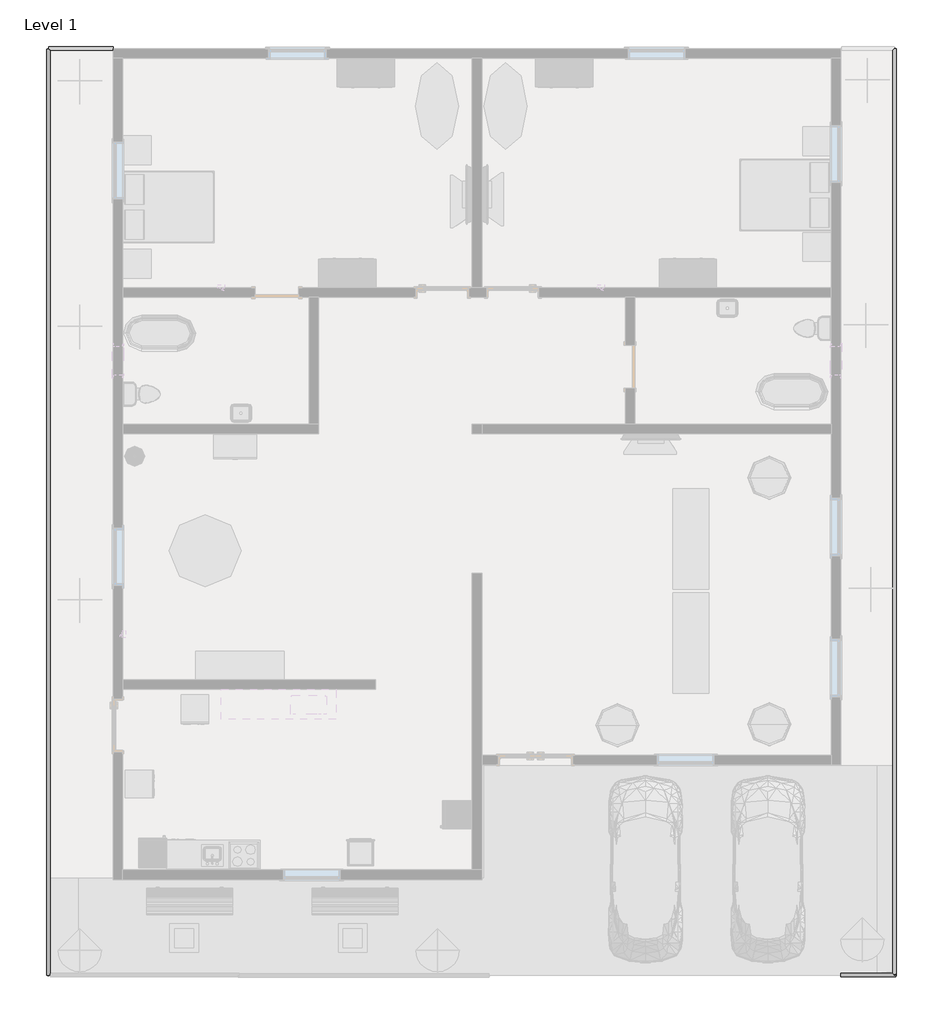
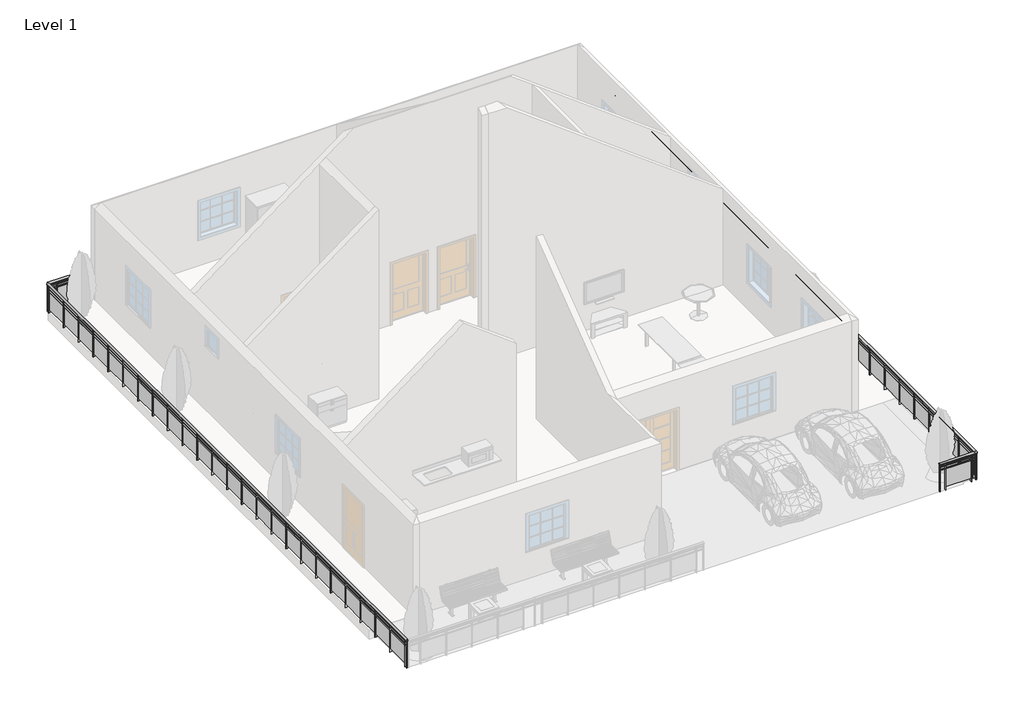
# One storey, part 2 of 3: 4 railings.
"""IFC4 building model written with IfcOpenShell, lengths in millimetres."""

from ifc_helpers import new_model, si_unit, point, frame, origin, origin_with_axes, place, context, project, spatial, polyline, ellipse_curve, trimmed, outline, extrude, element, save
from ifc_brep_helpers import plane_surface, extruded_surface, advanced_brep

model = new_model("IFC4")

# Units and contexts
model_context = context("Model", 3, world=origin())
ifc_project = project(units=[si_unit("LENGTHUNIT", "METRE", prefix="MILLI")], contexts=[model_context])

# Site, building, storey
site = spatial("IfcSite", under=ifc_project)
building = spatial("IfcBuilding", under=site)
storey = spatial("IfcBuildingStorey", under=building, Name="Level 1", Elevation=0.0)

# Railings
placement = place(None, origin())
element("IfcRailing", 1, ObjectType="Glass Panel - Bottom Fill", at=placement, inside=storey, context=model_context, shape_type="SolidModel", body=[
    advanced_brep(
    [(-18419.9392853, 13548.4299175, 914.4), (-18496.1392853, 13548.4299175, 914.4), (-18419.9392853, -6127.0450825, 914.4), (-18496.1392853, -6127.0450825, 914.4)],
    [
        (0, 1, ellipse_curve(frame((-18458.0392853, 13548.4299175, 914.4), z_axis=(0.0, 1.0, 0.0), x_axis=(-1.0, 0.0, 0.0)), 38.1, 28.575)),
        (1, 0, ellipse_curve(frame((-18458.0392853, 13548.4299175, 914.4), z_axis=(0.0, 1.0, 0.0), x_axis=(-1.0, 0.0, 0.0)), 38.1, 28.575)),
        (2, 3, ellipse_curve(frame((-18458.0392853, -6127.0450825, 914.4), z_axis=(0.0, -1.0, 0.0), x_axis=(-1.0, 0.0, 0.0)), 38.1, 28.575)),
        (3, 2, ellipse_curve(frame((-18458.0392853, -6127.0450825, 914.4), z_axis=(0.0, -1.0, 0.0), x_axis=(-1.0, 0.0, 0.0)), 38.1, 28.575)),
        (0, 2),
        (3, 1),
    ],
    [
        plane_surface(frame((-18458.0392853, 13548.4299175, 914.4), z_axis=(0.0, 1.0, 0.0), x_axis=(0.0, 0.0, -1.0))),
        plane_surface(frame((-18458.0392853, -6127.0450825, 914.4), z_axis=(0.0, -1.0, 0.0), x_axis=(0.0, 0.0, -1.0))),
        extruded_surface(trimmed(ellipse_curve(frame((-18458.0392853, -6127.0450825, 914.4), z_axis=(0.0, 1.0, 0.0), x_axis=(-1.0, 0.0, 0.0)), 38.1, 28.575), [point((-18419.9392853, -6127.0450825, 914.4))], [point((-18496.1392853, -6127.0450825, 914.4))], True, "CARTESIAN"), (0.0, 19675.475, 0.0), 19675.475),
        extruded_surface(trimmed(ellipse_curve(frame((-18458.0392853, -6127.0450825, 914.4), z_axis=(0.0, 1.0, 0.0), x_axis=(-1.0, 0.0, 0.0)), 38.1, 28.575), [point((-18496.1392853, -6127.0450825, 914.4))], [point((-18419.9392853, -6127.0450825, 914.4))], True, "CARTESIAN"), (0.0, 19675.475, 0.0), 19675.475),
    ],
    [
        (0, [[1, 2]]),
        (1, [[3, 4]]),
        (2, [[-1, 5, -4, 6]]),
        (3, [[-2, -6, -3, -5]]),
    ],
),
    extrude(outline(polyline([(-18470.7392853, 13548.4299175), (-18445.3392853, 13548.4299175), (-18445.3392853, -6127.0450825), (-18470.7392853, -6127.0450825), (-18470.7392853, 13548.4299175)])), frame((0.0, 0.0, 800.1), z_axis=(0.0, 0.0, 1.0), x_axis=(1.0, 0.0, 0.0)), (0.0, 0.0, 1.0), 25.4),
    extrude(outline(polyline([(-18470.7392853, 13548.4299175), (-18445.3392853, 13548.4299175), (-18445.3392853, -6127.0450825), (-18470.7392853, -6127.0450825), (-18470.7392853, 13548.4299175)])), frame((0.0, 0.0, 698.5), z_axis=(0.0, 0.0, 1.0), x_axis=(1.0, 0.0, 0.0)), (0.0, 0.0, 1.0), 25.4),
    extrude(outline(polyline([(-18483.4392853, -6036.5575825), (-18432.6392853, -6036.5575825), (-18432.6392853, -6049.2575825), (-18483.4392853, -6049.2575825), (-18483.4392853, -6036.5575825)])), origin_with_axes(), (0.0, 0.0, 1.0), 885.6788223),
    extrude(outline(polyline([(-18451.5041283, -5230.1075825), (-18451.5041283, -6042.9075825), (-18457.8541283, -6042.9075825), (-18457.8541283, -5230.1075825), (-18451.5041283, -5230.1075825)])), frame((0.0, 0.0, 101.6), z_axis=(0.0, 0.0, 1.0), x_axis=(1.0, 0.0, 0.0)), (0.0, 0.0, 1.0), 596.9),
    extrude(outline(polyline([(-18483.4392853, -5223.7575825), (-18432.6392853, -5223.7575825), (-18432.6392853, -5236.4575825), (-18483.4392853, -5236.4575825), (-18483.4392853, -5223.7575825)])), origin_with_axes(), (0.0, 0.0, 1.0), 885.6788223),
    extrude(outline(polyline([(-18451.5041283, -4417.3075825), (-18451.5041283, -5230.1075825), (-18457.8541283, -5230.1075825), (-18457.8541283, -4417.3075825), (-18451.5041283, -4417.3075825)])), frame((0.0, 0.0, 101.6), z_axis=(0.0, 0.0, 1.0), x_axis=(1.0, 0.0, 0.0)), (0.0, 0.0, 1.0), 596.9),
    extrude(outline(polyline([(-18483.4392853, -4410.9575825), (-18432.6392853, -4410.9575825), (-18432.6392853, -4423.6575825), (-18483.4392853, -4423.6575825), (-18483.4392853, -4410.9575825)])), origin_with_axes(), (0.0, 0.0, 1.0), 885.6788223),
    extrude(outline(polyline([(-18451.5041283, -3604.5075825), (-18451.5041283, -4417.3075825), (-18457.8541283, -4417.3075825), (-18457.8541283, -3604.5075825), (-18451.5041283, -3604.5075825)])), frame((0.0, 0.0, 101.6), z_axis=(0.0, 0.0, 1.0), x_axis=(1.0, 0.0, 0.0)), (0.0, 0.0, 1.0), 596.9),
    extrude(outline(polyline([(-18483.4392853, -3598.1575825), (-18432.6392853, -3598.1575825), (-18432.6392853, -3610.8575825), (-18483.4392853, -3610.8575825), (-18483.4392853, -3598.1575825)])), origin_with_axes(), (0.0, 0.0, 1.0), 885.6788223),
    extrude(outline(polyline([(-18451.5041283, -2791.7075825), (-18451.5041283, -3604.5075825), (-18457.8541283, -3604.5075825), (-18457.8541283, -2791.7075825), (-18451.5041283, -2791.7075825)])), frame((0.0, 0.0, 101.6), z_axis=(0.0, 0.0, 1.0), x_axis=(1.0, 0.0, 0.0)), (0.0, 0.0, 1.0), 596.9),
    extrude(outline(polyline([(-18483.4392853, -2785.3575825), (-18432.6392853, -2785.3575825), (-18432.6392853, -2798.0575825), (-18483.4392853, -2798.0575825), (-18483.4392853, -2785.3575825)])), origin_with_axes(), (0.0, 0.0, 1.0), 885.6788223),
    extrude(outline(polyline([(-18451.5041283, -1978.9075825), (-18451.5041283, -2791.7075825), (-18457.8541283, -2791.7075825), (-18457.8541283, -1978.9075825), (-18451.5041283, -1978.9075825)])), frame((0.0, 0.0, 101.6), z_axis=(0.0, 0.0, 1.0), x_axis=(1.0, 0.0, 0.0)), (0.0, 0.0, 1.0), 596.9),
    extrude(outline(polyline([(-18483.4392853, -1972.5575825), (-18432.6392853, -1972.5575825), (-18432.6392853, -1985.2575825), (-18483.4392853, -1985.2575825), (-18483.4392853, -1972.5575825)])), origin_with_axes(), (0.0, 0.0, 1.0), 885.6788223),
    extrude(outline(polyline([(-18451.5041283, -1166.1075825), (-18451.5041283, -1978.9075825), (-18457.8541283, -1978.9075825), (-18457.8541283, -1166.1075825), (-18451.5041283, -1166.1075825)])), frame((0.0, 0.0, 101.6), z_axis=(0.0, 0.0, 1.0), x_axis=(1.0, 0.0, 0.0)), (0.0, 0.0, 1.0), 596.9),
    extrude(outline(polyline([(-18483.4392853, -1159.7575825), (-18432.6392853, -1159.7575825), (-18432.6392853, -1172.4575825), (-18483.4392853, -1172.4575825), (-18483.4392853, -1159.7575825)])), origin_with_axes(), (0.0, 0.0, 1.0), 885.6788223),
    extrude(outline(polyline([(-18451.5041283, -353.3075825), (-18451.5041283, -1166.1075825), (-18457.8541283, -1166.1075825), (-18457.8541283, -353.3075825), (-18451.5041283, -353.3075825)])), frame((0.0, 0.0, 101.6), z_axis=(0.0, 0.0, 1.0), x_axis=(1.0, 0.0, 0.0)), (0.0, 0.0, 1.0), 596.9),
    extrude(outline(polyline([(-18483.4392853, -346.9575825), (-18432.6392853, -346.9575825), (-18432.6392853, -359.6575825), (-18483.4392853, -359.6575825), (-18483.4392853, -346.9575825)])), origin_with_axes(), (0.0, 0.0, 1.0), 885.6788223),
    extrude(outline(polyline([(-18451.5041283, 459.4924175), (-18451.5041283, -353.3075825), (-18457.8541283, -353.3075825), (-18457.8541283, 459.4924175), (-18451.5041283, 459.4924175)])), frame((0.0, 0.0, 101.6), z_axis=(0.0, 0.0, 1.0), x_axis=(1.0, 0.0, 0.0)), (0.0, 0.0, 1.0), 596.9),
    extrude(outline(polyline([(-18483.4392853, 465.8424175), (-18432.6392853, 465.8424175), (-18432.6392853, 453.1424175), (-18483.4392853, 453.1424175), (-18483.4392853, 465.8424175)])), origin_with_axes(), (0.0, 0.0, 1.0), 885.6788223),
    extrude(outline(polyline([(-18451.5041283, 1272.2924175), (-18451.5041283, 459.4924175), (-18457.8541283, 459.4924175), (-18457.8541283, 1272.2924175), (-18451.5041283, 1272.2924175)])), frame((0.0, 0.0, 101.6), z_axis=(0.0, 0.0, 1.0), x_axis=(1.0, 0.0, 0.0)), (0.0, 0.0, 1.0), 596.9),
    extrude(outline(polyline([(-18483.4392853, 1278.6424175), (-18432.6392853, 1278.6424175), (-18432.6392853, 1265.9424175), (-18483.4392853, 1265.9424175), (-18483.4392853, 1278.6424175)])), origin_with_axes(), (0.0, 0.0, 1.0), 885.6788223),
    extrude(outline(polyline([(-18451.5041283, 2085.0924175), (-18451.5041283, 1272.2924175), (-18457.8541283, 1272.2924175), (-18457.8541283, 2085.0924175), (-18451.5041283, 2085.0924175)])), frame((0.0, 0.0, 101.6), z_axis=(0.0, 0.0, 1.0), x_axis=(1.0, 0.0, 0.0)), (0.0, 0.0, 1.0), 596.9),
    extrude(outline(polyline([(-18483.4392853, 2091.4424175), (-18432.6392853, 2091.4424175), (-18432.6392853, 2078.7424175), (-18483.4392853, 2078.7424175), (-18483.4392853, 2091.4424175)])), origin_with_axes(), (0.0, 0.0, 1.0), 885.6788223),
    extrude(outline(polyline([(-18451.5041283, 2897.8924175), (-18451.5041283, 2085.0924175), (-18457.8541283, 2085.0924175), (-18457.8541283, 2897.8924175), (-18451.5041283, 2897.8924175)])), frame((0.0, 0.0, 101.6), z_axis=(0.0, 0.0, 1.0), x_axis=(1.0, 0.0, 0.0)), (0.0, 0.0, 1.0), 596.9),
    extrude(outline(polyline([(-18483.4392853, 2904.2424175), (-18432.6392853, 2904.2424175), (-18432.6392853, 2891.5424175), (-18483.4392853, 2891.5424175), (-18483.4392853, 2904.2424175)])), origin_with_axes(), (0.0, 0.0, 1.0), 885.6788223),
    extrude(outline(polyline([(-18451.5041283, 3710.6924175), (-18451.5041283, 2897.8924175), (-18457.8541283, 2897.8924175), (-18457.8541283, 3710.6924175), (-18451.5041283, 3710.6924175)])), frame((0.0, 0.0, 101.6), z_axis=(0.0, 0.0, 1.0), x_axis=(1.0, 0.0, 0.0)), (0.0, 0.0, 1.0), 596.9),
    extrude(outline(polyline([(-18483.4392853, 3717.0424175), (-18432.6392853, 3717.0424175), (-18432.6392853, 3704.3424175), (-18483.4392853, 3704.3424175), (-18483.4392853, 3717.0424175)])), origin_with_axes(), (0.0, 0.0, 1.0), 885.6788223),
    extrude(outline(polyline([(-18451.5041283, 4523.4924175), (-18451.5041283, 3710.6924175), (-18457.8541283, 3710.6924175), (-18457.8541283, 4523.4924175), (-18451.5041283, 4523.4924175)])), frame((0.0, 0.0, 101.6), z_axis=(0.0, 0.0, 1.0), x_axis=(1.0, 0.0, 0.0)), (0.0, 0.0, 1.0), 596.9),
    extrude(outline(polyline([(-18483.4392853, 4529.8424175), (-18432.6392853, 4529.8424175), (-18432.6392853, 4517.1424175), (-18483.4392853, 4517.1424175), (-18483.4392853, 4529.8424175)])), origin_with_axes(), (0.0, 0.0, 1.0), 885.6788223),
    extrude(outline(polyline([(-18451.5041283, 5336.2924175), (-18451.5041283, 4523.4924175), (-18457.8541283, 4523.4924175), (-18457.8541283, 5336.2924175), (-18451.5041283, 5336.2924175)])), frame((0.0, 0.0, 101.6), z_axis=(0.0, 0.0, 1.0), x_axis=(1.0, 0.0, 0.0)), (0.0, 0.0, 1.0), 596.9),
    extrude(outline(polyline([(-18483.4392853, 5342.6424175), (-18432.6392853, 5342.6424175), (-18432.6392853, 5329.9424175), (-18483.4392853, 5329.9424175), (-18483.4392853, 5342.6424175)])), origin_with_axes(), (0.0, 0.0, 1.0), 885.6788223),
    extrude(outline(polyline([(-18451.5041283, 6149.0924175), (-18451.5041283, 5336.2924175), (-18457.8541283, 5336.2924175), (-18457.8541283, 6149.0924175), (-18451.5041283, 6149.0924175)])), frame((0.0, 0.0, 101.6), z_axis=(0.0, 0.0, 1.0), x_axis=(1.0, 0.0, 0.0)), (0.0, 0.0, 1.0), 596.9),
    extrude(outline(polyline([(-18483.4392853, 6155.4424175), (-18432.6392853, 6155.4424175), (-18432.6392853, 6142.7424175), (-18483.4392853, 6142.7424175), (-18483.4392853, 6155.4424175)])), origin_with_axes(), (0.0, 0.0, 1.0), 885.6788223),
    extrude(outline(polyline([(-18451.5041283, 6961.8924175), (-18451.5041283, 6149.0924175), (-18457.8541283, 6149.0924175), (-18457.8541283, 6961.8924175), (-18451.5041283, 6961.8924175)])), frame((0.0, 0.0, 101.6), z_axis=(0.0, 0.0, 1.0), x_axis=(1.0, 0.0, 0.0)), (0.0, 0.0, 1.0), 596.9),
    extrude(outline(polyline([(-18483.4392853, 6968.2424175), (-18432.6392853, 6968.2424175), (-18432.6392853, 6955.5424175), (-18483.4392853, 6955.5424175), (-18483.4392853, 6968.2424175)])), origin_with_axes(), (0.0, 0.0, 1.0), 885.6788223),
    extrude(outline(polyline([(-18451.5041283, 7774.6924175), (-18451.5041283, 6961.8924175), (-18457.8541283, 6961.8924175), (-18457.8541283, 7774.6924175), (-18451.5041283, 7774.6924175)])), frame((0.0, 0.0, 101.6), z_axis=(0.0, 0.0, 1.0), x_axis=(1.0, 0.0, 0.0)), (0.0, 0.0, 1.0), 596.9),
    extrude(outline(polyline([(-18483.4392853, 7781.0424175), (-18432.6392853, 7781.0424175), (-18432.6392853, 7768.3424175), (-18483.4392853, 7768.3424175), (-18483.4392853, 7781.0424175)])), origin_with_axes(), (0.0, 0.0, 1.0), 885.6788223),
    extrude(outline(polyline([(-18451.5041283, 8587.4924175), (-18451.5041283, 7774.6924175), (-18457.8541283, 7774.6924175), (-18457.8541283, 8587.4924175), (-18451.5041283, 8587.4924175)])), frame((0.0, 0.0, 101.6), z_axis=(0.0, 0.0, 1.0), x_axis=(1.0, 0.0, 0.0)), (0.0, 0.0, 1.0), 596.9),
    extrude(outline(polyline([(-18483.4392853, 8593.8424175), (-18432.6392853, 8593.8424175), (-18432.6392853, 8581.1424175), (-18483.4392853, 8581.1424175), (-18483.4392853, 8593.8424175)])), origin_with_axes(), (0.0, 0.0, 1.0), 885.6788223),
    extrude(outline(polyline([(-18451.5041283, 9400.2924175), (-18451.5041283, 8587.4924175), (-18457.8541283, 8587.4924175), (-18457.8541283, 9400.2924175), (-18451.5041283, 9400.2924175)])), frame((0.0, 0.0, 101.6), z_axis=(0.0, 0.0, 1.0), x_axis=(1.0, 0.0, 0.0)), (0.0, 0.0, 1.0), 596.9),
    extrude(outline(polyline([(-18483.4392853, 9406.6424175), (-18432.6392853, 9406.6424175), (-18432.6392853, 9393.9424175), (-18483.4392853, 9393.9424175), (-18483.4392853, 9406.6424175)])), origin_with_axes(), (0.0, 0.0, 1.0), 885.6788223),
    extrude(outline(polyline([(-18451.5041283, 10213.0924175), (-18451.5041283, 9400.2924175), (-18457.8541283, 9400.2924175), (-18457.8541283, 10213.0924175), (-18451.5041283, 10213.0924175)])), frame((0.0, 0.0, 101.6), z_axis=(0.0, 0.0, 1.0), x_axis=(1.0, 0.0, 0.0)), (0.0, 0.0, 1.0), 596.9),
    extrude(outline(polyline([(-18483.4392853, 10219.4424175), (-18432.6392853, 10219.4424175), (-18432.6392853, 10206.7424175), (-18483.4392853, 10206.7424175), (-18483.4392853, 10219.4424175)])), origin_with_axes(), (0.0, 0.0, 1.0), 885.6788223),
    extrude(outline(polyline([(-18451.5041283, 11025.8924175), (-18451.5041283, 10213.0924175), (-18457.8541283, 10213.0924175), (-18457.8541283, 11025.8924175), (-18451.5041283, 11025.8924175)])), frame((0.0, 0.0, 101.6), z_axis=(0.0, 0.0, 1.0), x_axis=(1.0, 0.0, 0.0)), (0.0, 0.0, 1.0), 596.9),
    extrude(outline(polyline([(-18483.4392853, 11032.2424175), (-18432.6392853, 11032.2424175), (-18432.6392853, 11019.5424175), (-18483.4392853, 11019.5424175), (-18483.4392853, 11032.2424175)])), origin_with_axes(), (0.0, 0.0, 1.0), 885.6788223),
    extrude(outline(polyline([(-18451.5041283, 11838.6924175), (-18451.5041283, 11025.8924175), (-18457.8541283, 11025.8924175), (-18457.8541283, 11838.6924175), (-18451.5041283, 11838.6924175)])), frame((0.0, 0.0, 101.6), z_axis=(0.0, 0.0, 1.0), x_axis=(1.0, 0.0, 0.0)), (0.0, 0.0, 1.0), 596.9),
    extrude(outline(polyline([(-18483.4392853, 11845.0424175), (-18432.6392853, 11845.0424175), (-18432.6392853, 11832.3424175), (-18483.4392853, 11832.3424175), (-18483.4392853, 11845.0424175)])), origin_with_axes(), (0.0, 0.0, 1.0), 885.6788223),
    extrude(outline(polyline([(-18451.5041283, 12651.4924175), (-18451.5041283, 11838.6924175), (-18457.8541283, 11838.6924175), (-18457.8541283, 12651.4924175), (-18451.5041283, 12651.4924175)])), frame((0.0, 0.0, 101.6), z_axis=(0.0, 0.0, 1.0), x_axis=(1.0, 0.0, 0.0)), (0.0, 0.0, 1.0), 596.9),
    extrude(outline(polyline([(-18483.4392853, 12657.8424175), (-18432.6392853, 12657.8424175), (-18432.6392853, 12645.1424175), (-18483.4392853, 12645.1424175), (-18483.4392853, 12657.8424175)])), origin_with_axes(), (0.0, 0.0, 1.0), 885.6788223),
    extrude(outline(polyline([(-18451.5041283, 13464.2924175), (-18451.5041283, 12651.4924175), (-18457.8541283, 12651.4924175), (-18457.8541283, 13464.2924175), (-18451.5041283, 13464.2924175)])), frame((0.0, 0.0, 101.6), z_axis=(0.0, 0.0, 1.0), x_axis=(1.0, 0.0, 0.0)), (0.0, 0.0, 1.0), 596.9),
    extrude(outline(polyline([(-18483.4392853, 13470.6424175), (-18432.6392853, 13470.6424175), (-18432.6392853, 13457.9424175), (-18483.4392853, 13457.9424175), (-18483.4392853, 13470.6424175)])), origin_with_axes(), (0.0, 0.0, 1.0), 885.6788223),
    extrude(outline(polyline([(-18467.5642853, -6114.3450825), (-18448.5142853, -6114.3450825), (-18448.5142853, -6133.3950825), (-18467.5642853, -6133.3950825), (-18467.5642853, -6114.3450825)])), origin_with_axes(), (0.0, 0.0, 1.0), 885.6788223),
    extrude(outline(polyline([(-18467.5642853, 13554.7799175), (-18448.5142853, 13554.7799175), (-18448.5142853, 13535.7299175), (-18467.5642853, 13535.7299175), (-18467.5642853, 13554.7799175)])), origin_with_axes(), (0.0, 0.0, 1.0), 885.6788223),
])
element("IfcRailing", 2, ObjectType="Glass Panel - Bottom Fill", at=placement, inside=storey, context=model_context, shape_type="SolidModel", body=[
    advanced_brep(
    [(-506.5892853, -6127.0450825, 914.4), (-430.3892853, -6127.0450825, 914.4), (-506.5892853, 13557.9549175, 914.4), (-430.3892853, 13557.9549175, 914.4)],
    [
        (0, 1, ellipse_curve(frame((-468.4892853, -6127.0450825, 914.4), z_axis=(0.0, -1.0, 0.0), x_axis=(1.0, 0.0, 0.0)), 38.1, 28.575)),
        (1, 0, ellipse_curve(frame((-468.4892853, -6127.0450825, 914.4), z_axis=(0.0, -1.0, 0.0), x_axis=(1.0, 0.0, 0.0)), 38.1, 28.575)),
        (2, 3, ellipse_curve(frame((-468.4892853, 13557.9549175, 914.4), z_axis=(0.0, 1.0, 0.0), x_axis=(1.0, 0.0, 0.0)), 38.1, 28.575)),
        (3, 2, ellipse_curve(frame((-468.4892853, 13557.9549175, 914.4), z_axis=(0.0, 1.0, 0.0), x_axis=(1.0, 0.0, 0.0)), 38.1, 28.575)),
        (0, 2),
        (3, 1),
    ],
    [
        plane_surface(frame((-468.4892853, -6127.0450825, 914.4), z_axis=(0.0, -1.0, 0.0), x_axis=(0.0, 0.0, 1.0))),
        plane_surface(frame((-468.4892853, 13557.9549175, 914.4), z_axis=(0.0, 1.0, 0.0), x_axis=(0.0, 0.0, 1.0))),
        extruded_surface(trimmed(ellipse_curve(frame((-468.4892853, 13557.9549175, 914.4), z_axis=(0.0, -1.0, 0.0), x_axis=(1.0, 0.0, 0.0)), 38.1, 28.575), [point((-506.5892853, 13557.9549175, 914.4))], [point((-430.3892853, 13557.9549175, 914.4))], True, "CARTESIAN"), (0.0, -19685.0, 0.0), 19685.0),
        extruded_surface(trimmed(ellipse_curve(frame((-468.4892853, 13557.9549175, 914.4), z_axis=(0.0, -1.0, 0.0), x_axis=(1.0, 0.0, 0.0)), 38.1, 28.575), [point((-430.3892853, 13557.9549175, 914.4))], [point((-506.5892853, 13557.9549175, 914.4))], True, "CARTESIAN"), (0.0, -19685.0, 0.0), 19685.0),
    ],
    [
        (0, [[1, 2]]),
        (1, [[3, 4]]),
        (2, [[-1, 5, -4, 6]]),
        (3, [[-2, -6, -3, -5]]),
    ],
),
    extrude(outline(polyline([(-455.7892853, -6127.0450825), (-481.1892853, -6127.0450825), (-481.1892853, 13557.9549175), (-455.7892853, 13557.9549175), (-455.7892853, -6127.0450825)])), frame((0.0, 0.0, 800.1), z_axis=(0.0, 0.0, 1.0), x_axis=(1.0, 0.0, 0.0)), (0.0, 0.0, 1.0), 25.4),
    extrude(outline(polyline([(-455.7892853, -6127.0450825), (-481.1892853, -6127.0450825), (-481.1892853, 13557.9549175), (-455.7892853, 13557.9549175), (-455.7892853, -6127.0450825)])), frame((0.0, 0.0, 698.5), z_axis=(0.0, 0.0, 1.0), x_axis=(1.0, 0.0, 0.0)), (0.0, 0.0, 1.0), 25.4),
    extrude(outline(polyline([(-493.8892853, 13462.7049175), (-493.8892853, 13475.4049175), (-443.0892853, 13475.4049175), (-443.0892853, 13462.7049175), (-493.8892853, 13462.7049175)])), origin_with_axes(), (0.0, 0.0, 1.0), 885.6788223),
    extrude(outline(polyline([(-461.9541283, 12656.2549175), (-468.3041283, 12656.2549175), (-468.3041283, 13469.0549175), (-461.9541283, 13469.0549175), (-461.9541283, 12656.2549175)])), frame((0.0, 0.0, 101.6), z_axis=(0.0, 0.0, 1.0), x_axis=(1.0, 0.0, 0.0)), (0.0, 0.0, 1.0), 596.9),
    extrude(outline(polyline([(-493.8892853, 12649.9049175), (-493.8892853, 12662.6049175), (-443.0892853, 12662.6049175), (-443.0892853, 12649.9049175), (-493.8892853, 12649.9049175)])), origin_with_axes(), (0.0, 0.0, 1.0), 885.6788223),
    extrude(outline(polyline([(-461.9541283, 11843.4549175), (-468.3041283, 11843.4549175), (-468.3041283, 12656.2549175), (-461.9541283, 12656.2549175), (-461.9541283, 11843.4549175)])), frame((0.0, 0.0, 101.6), z_axis=(0.0, 0.0, 1.0), x_axis=(1.0, 0.0, 0.0)), (0.0, 0.0, 1.0), 596.9),
    extrude(outline(polyline([(-493.8892853, 11837.1049175), (-493.8892853, 11849.8049175), (-443.0892853, 11849.8049175), (-443.0892853, 11837.1049175), (-493.8892853, 11837.1049175)])), origin_with_axes(), (0.0, 0.0, 1.0), 885.6788223),
    extrude(outline(polyline([(-461.9541283, 11030.6549175), (-468.3041283, 11030.6549175), (-468.3041283, 11843.4549175), (-461.9541283, 11843.4549175), (-461.9541283, 11030.6549175)])), frame((0.0, 0.0, 101.6), z_axis=(0.0, 0.0, 1.0), x_axis=(1.0, 0.0, 0.0)), (0.0, 0.0, 1.0), 596.9),
    extrude(outline(polyline([(-493.8892853, 11024.3049175), (-493.8892853, 11037.0049175), (-443.0892853, 11037.0049175), (-443.0892853, 11024.3049175), (-493.8892853, 11024.3049175)])), origin_with_axes(), (0.0, 0.0, 1.0), 885.6788223),
    extrude(outline(polyline([(-461.9541283, 10217.8549175), (-468.3041283, 10217.8549175), (-468.3041283, 11030.6549175), (-461.9541283, 11030.6549175), (-461.9541283, 10217.8549175)])), frame((0.0, 0.0, 101.6), z_axis=(0.0, 0.0, 1.0), x_axis=(1.0, 0.0, 0.0)), (0.0, 0.0, 1.0), 596.9),
    extrude(outline(polyline([(-493.8892853, 10211.5049175), (-493.8892853, 10224.2049175), (-443.0892853, 10224.2049175), (-443.0892853, 10211.5049175), (-493.8892853, 10211.5049175)])), origin_with_axes(), (0.0, 0.0, 1.0), 885.6788223),
    extrude(outline(polyline([(-461.9541283, 9405.0549175), (-468.3041283, 9405.0549175), (-468.3041283, 10217.8549175), (-461.9541283, 10217.8549175), (-461.9541283, 9405.0549175)])), frame((0.0, 0.0, 101.6), z_axis=(0.0, 0.0, 1.0), x_axis=(1.0, 0.0, 0.0)), (0.0, 0.0, 1.0), 596.9),
    extrude(outline(polyline([(-493.8892853, 9398.7049175), (-493.8892853, 9411.4049175), (-443.0892853, 9411.4049175), (-443.0892853, 9398.7049175), (-493.8892853, 9398.7049175)])), origin_with_axes(), (0.0, 0.0, 1.0), 885.6788223),
    extrude(outline(polyline([(-461.9541283, 8592.2549175), (-468.3041283, 8592.2549175), (-468.3041283, 9405.0549175), (-461.9541283, 9405.0549175), (-461.9541283, 8592.2549175)])), frame((0.0, 0.0, 101.6), z_axis=(0.0, 0.0, 1.0), x_axis=(1.0, 0.0, 0.0)), (0.0, 0.0, 1.0), 596.9),
    extrude(outline(polyline([(-493.8892853, 8585.9049175), (-493.8892853, 8598.6049175), (-443.0892853, 8598.6049175), (-443.0892853, 8585.9049175), (-493.8892853, 8585.9049175)])), origin_with_axes(), (0.0, 0.0, 1.0), 885.6788223),
    extrude(outline(polyline([(-461.9541283, 7779.4549175), (-468.3041283, 7779.4549175), (-468.3041283, 8592.2549175), (-461.9541283, 8592.2549175), (-461.9541283, 7779.4549175)])), frame((0.0, 0.0, 101.6), z_axis=(0.0, 0.0, 1.0), x_axis=(1.0, 0.0, 0.0)), (0.0, 0.0, 1.0), 596.9),
    extrude(outline(polyline([(-493.8892853, 7773.1049175), (-493.8892853, 7785.8049175), (-443.0892853, 7785.8049175), (-443.0892853, 7773.1049175), (-493.8892853, 7773.1049175)])), origin_with_axes(), (0.0, 0.0, 1.0), 885.6788223),
    extrude(outline(polyline([(-461.9541283, 6966.6549175), (-468.3041283, 6966.6549175), (-468.3041283, 7779.4549175), (-461.9541283, 7779.4549175), (-461.9541283, 6966.6549175)])), frame((0.0, 0.0, 101.6), z_axis=(0.0, 0.0, 1.0), x_axis=(1.0, 0.0, 0.0)), (0.0, 0.0, 1.0), 596.9),
    extrude(outline(polyline([(-493.8892853, 6960.3049175), (-493.8892853, 6973.0049175), (-443.0892853, 6973.0049175), (-443.0892853, 6960.3049175), (-493.8892853, 6960.3049175)])), origin_with_axes(), (0.0, 0.0, 1.0), 885.6788223),
    extrude(outline(polyline([(-461.9541283, 6153.8549175), (-468.3041283, 6153.8549175), (-468.3041283, 6966.6549175), (-461.9541283, 6966.6549175), (-461.9541283, 6153.8549175)])), frame((0.0, 0.0, 101.6), z_axis=(0.0, 0.0, 1.0), x_axis=(1.0, 0.0, 0.0)), (0.0, 0.0, 1.0), 596.9),
    extrude(outline(polyline([(-493.8892853, 6147.5049175), (-493.8892853, 6160.2049175), (-443.0892853, 6160.2049175), (-443.0892853, 6147.5049175), (-493.8892853, 6147.5049175)])), origin_with_axes(), (0.0, 0.0, 1.0), 885.6788223),
    extrude(outline(polyline([(-461.9541283, 5341.0549175), (-468.3041283, 5341.0549175), (-468.3041283, 6153.8549175), (-461.9541283, 6153.8549175), (-461.9541283, 5341.0549175)])), frame((0.0, 0.0, 101.6), z_axis=(0.0, 0.0, 1.0), x_axis=(1.0, 0.0, 0.0)), (0.0, 0.0, 1.0), 596.9),
    extrude(outline(polyline([(-493.8892853, 5334.7049175), (-493.8892853, 5347.4049175), (-443.0892853, 5347.4049175), (-443.0892853, 5334.7049175), (-493.8892853, 5334.7049175)])), origin_with_axes(), (0.0, 0.0, 1.0), 885.6788223),
    extrude(outline(polyline([(-461.9541283, 4528.2549175), (-468.3041283, 4528.2549175), (-468.3041283, 5341.0549175), (-461.9541283, 5341.0549175), (-461.9541283, 4528.2549175)])), frame((0.0, 0.0, 101.6), z_axis=(0.0, 0.0, 1.0), x_axis=(1.0, 0.0, 0.0)), (0.0, 0.0, 1.0), 596.9),
    extrude(outline(polyline([(-493.8892853, 4521.9049175), (-493.8892853, 4534.6049175), (-443.0892853, 4534.6049175), (-443.0892853, 4521.9049175), (-493.8892853, 4521.9049175)])), origin_with_axes(), (0.0, 0.0, 1.0), 885.6788223),
    extrude(outline(polyline([(-461.9541283, 3715.4549175), (-468.3041283, 3715.4549175), (-468.3041283, 4528.2549175), (-461.9541283, 4528.2549175), (-461.9541283, 3715.4549175)])), frame((0.0, 0.0, 101.6), z_axis=(0.0, 0.0, 1.0), x_axis=(1.0, 0.0, 0.0)), (0.0, 0.0, 1.0), 596.9),
    extrude(outline(polyline([(-493.8892853, 3709.1049175), (-493.8892853, 3721.8049175), (-443.0892853, 3721.8049175), (-443.0892853, 3709.1049175), (-493.8892853, 3709.1049175)])), origin_with_axes(), (0.0, 0.0, 1.0), 885.6788223),
    extrude(outline(polyline([(-461.9541283, 2902.6549175), (-468.3041283, 2902.6549175), (-468.3041283, 3715.4549175), (-461.9541283, 3715.4549175), (-461.9541283, 2902.6549175)])), frame((0.0, 0.0, 101.6), z_axis=(0.0, 0.0, 1.0), x_axis=(1.0, 0.0, 0.0)), (0.0, 0.0, 1.0), 596.9),
    extrude(outline(polyline([(-493.8892853, 2896.3049175), (-493.8892853, 2909.0049175), (-443.0892853, 2909.0049175), (-443.0892853, 2896.3049175), (-493.8892853, 2896.3049175)])), origin_with_axes(), (0.0, 0.0, 1.0), 885.6788223),
    extrude(outline(polyline([(-461.9541283, 2089.8549175), (-468.3041283, 2089.8549175), (-468.3041283, 2902.6549175), (-461.9541283, 2902.6549175), (-461.9541283, 2089.8549175)])), frame((0.0, 0.0, 101.6), z_axis=(0.0, 0.0, 1.0), x_axis=(1.0, 0.0, 0.0)), (0.0, 0.0, 1.0), 596.9),
    extrude(outline(polyline([(-493.8892853, 2083.5049175), (-493.8892853, 2096.2049175), (-443.0892853, 2096.2049175), (-443.0892853, 2083.5049175), (-493.8892853, 2083.5049175)])), origin_with_axes(), (0.0, 0.0, 1.0), 885.6788223),
    extrude(outline(polyline([(-461.9541283, 1277.0549175), (-468.3041283, 1277.0549175), (-468.3041283, 2089.8549175), (-461.9541283, 2089.8549175), (-461.9541283, 1277.0549175)])), frame((0.0, 0.0, 101.6), z_axis=(0.0, 0.0, 1.0), x_axis=(1.0, 0.0, 0.0)), (0.0, 0.0, 1.0), 596.9),
    extrude(outline(polyline([(-493.8892853, 1270.7049175), (-493.8892853, 1283.4049175), (-443.0892853, 1283.4049175), (-443.0892853, 1270.7049175), (-493.8892853, 1270.7049175)])), origin_with_axes(), (0.0, 0.0, 1.0), 885.6788223),
    extrude(outline(polyline([(-461.9541283, 464.2549175), (-468.3041283, 464.2549175), (-468.3041283, 1277.0549175), (-461.9541283, 1277.0549175), (-461.9541283, 464.2549175)])), frame((0.0, 0.0, 101.6), z_axis=(0.0, 0.0, 1.0), x_axis=(1.0, 0.0, 0.0)), (0.0, 0.0, 1.0), 596.9),
    extrude(outline(polyline([(-493.8892853, 457.9049175), (-493.8892853, 470.6049175), (-443.0892853, 470.6049175), (-443.0892853, 457.9049175), (-493.8892853, 457.9049175)])), origin_with_axes(), (0.0, 0.0, 1.0), 885.6788223),
    extrude(outline(polyline([(-461.9541283, -348.5450825), (-468.3041283, -348.5450825), (-468.3041283, 464.2549175), (-461.9541283, 464.2549175), (-461.9541283, -348.5450825)])), frame((0.0, 0.0, 101.6), z_axis=(0.0, 0.0, 1.0), x_axis=(1.0, 0.0, 0.0)), (0.0, 0.0, 1.0), 596.9),
    extrude(outline(polyline([(-493.8892853, -354.8950825), (-493.8892853, -342.1950825), (-443.0892853, -342.1950825), (-443.0892853, -354.8950825), (-493.8892853, -354.8950825)])), origin_with_axes(), (0.0, 0.0, 1.0), 885.6788223),
    extrude(outline(polyline([(-461.9541283, -1161.3450825), (-468.3041283, -1161.3450825), (-468.3041283, -348.5450825), (-461.9541283, -348.5450825), (-461.9541283, -1161.3450825)])), frame((0.0, 0.0, 101.6), z_axis=(0.0, 0.0, 1.0), x_axis=(1.0, 0.0, 0.0)), (0.0, 0.0, 1.0), 596.9),
    extrude(outline(polyline([(-493.8892853, -1167.6950825), (-493.8892853, -1154.9950825), (-443.0892853, -1154.9950825), (-443.0892853, -1167.6950825), (-493.8892853, -1167.6950825)])), origin_with_axes(), (0.0, 0.0, 1.0), 885.6788223),
    extrude(outline(polyline([(-461.9541283, -1974.1450825), (-468.3041283, -1974.1450825), (-468.3041283, -1161.3450825), (-461.9541283, -1161.3450825), (-461.9541283, -1974.1450825)])), frame((0.0, 0.0, 101.6), z_axis=(0.0, 0.0, 1.0), x_axis=(1.0, 0.0, 0.0)), (0.0, 0.0, 1.0), 596.9),
    extrude(outline(polyline([(-493.8892853, -1980.4950825), (-493.8892853, -1967.7950825), (-443.0892853, -1967.7950825), (-443.0892853, -1980.4950825), (-493.8892853, -1980.4950825)])), origin_with_axes(), (0.0, 0.0, 1.0), 885.6788223),
    extrude(outline(polyline([(-461.9541283, -2786.9450825), (-468.3041283, -2786.9450825), (-468.3041283, -1974.1450825), (-461.9541283, -1974.1450825), (-461.9541283, -2786.9450825)])), frame((0.0, 0.0, 101.6), z_axis=(0.0, 0.0, 1.0), x_axis=(1.0, 0.0, 0.0)), (0.0, 0.0, 1.0), 596.9),
    extrude(outline(polyline([(-493.8892853, -2793.2950825), (-493.8892853, -2780.5950825), (-443.0892853, -2780.5950825), (-443.0892853, -2793.2950825), (-493.8892853, -2793.2950825)])), origin_with_axes(), (0.0, 0.0, 1.0), 885.6788223),
    extrude(outline(polyline([(-461.9541283, -3599.7450825), (-468.3041283, -3599.7450825), (-468.3041283, -2786.9450825), (-461.9541283, -2786.9450825), (-461.9541283, -3599.7450825)])), frame((0.0, 0.0, 101.6), z_axis=(0.0, 0.0, 1.0), x_axis=(1.0, 0.0, 0.0)), (0.0, 0.0, 1.0), 596.9),
    extrude(outline(polyline([(-493.8892853, -3606.0950825), (-493.8892853, -3593.3950825), (-443.0892853, -3593.3950825), (-443.0892853, -3606.0950825), (-493.8892853, -3606.0950825)])), origin_with_axes(), (0.0, 0.0, 1.0), 885.6788223),
    extrude(outline(polyline([(-461.9541283, -4412.5450825), (-468.3041283, -4412.5450825), (-468.3041283, -3599.7450825), (-461.9541283, -3599.7450825), (-461.9541283, -4412.5450825)])), frame((0.0, 0.0, 101.6), z_axis=(0.0, 0.0, 1.0), x_axis=(1.0, 0.0, 0.0)), (0.0, 0.0, 1.0), 596.9),
    extrude(outline(polyline([(-493.8892853, -4418.8950825), (-493.8892853, -4406.1950825), (-443.0892853, -4406.1950825), (-443.0892853, -4418.8950825), (-493.8892853, -4418.8950825)])), origin_with_axes(), (0.0, 0.0, 1.0), 885.6788223),
    extrude(outline(polyline([(-461.9541283, -5225.3450825), (-468.3041283, -5225.3450825), (-468.3041283, -4412.5450825), (-461.9541283, -4412.5450825), (-461.9541283, -5225.3450825)])), frame((0.0, 0.0, 101.6), z_axis=(0.0, 0.0, 1.0), x_axis=(1.0, 0.0, 0.0)), (0.0, 0.0, 1.0), 596.9),
    extrude(outline(polyline([(-493.8892853, -5231.6950825), (-493.8892853, -5218.9950825), (-443.0892853, -5218.9950825), (-443.0892853, -5231.6950825), (-493.8892853, -5231.6950825)])), origin_with_axes(), (0.0, 0.0, 1.0), 885.6788223),
    extrude(outline(polyline([(-461.9541283, -6038.1450825), (-468.3041283, -6038.1450825), (-468.3041283, -5225.3450825), (-461.9541283, -5225.3450825), (-461.9541283, -6038.1450825)])), frame((0.0, 0.0, 101.6), z_axis=(0.0, 0.0, 1.0), x_axis=(1.0, 0.0, 0.0)), (0.0, 0.0, 1.0), 596.9),
    extrude(outline(polyline([(-493.8892853, -6044.4950825), (-493.8892853, -6031.7950825), (-443.0892853, -6031.7950825), (-443.0892853, -6044.4950825), (-493.8892853, -6044.4950825)])), origin_with_axes(), (0.0, 0.0, 1.0), 885.6788223),
    extrude(outline(polyline([(-478.0142853, 13545.2549175), (-478.0142853, 13564.3049175), (-458.9642853, 13564.3049175), (-458.9642853, 13545.2549175), (-478.0142853, 13545.2549175)])), origin_with_axes(), (0.0, 0.0, 1.0), 885.6788223),
    extrude(outline(polyline([(-478.0142853, -6133.3950825), (-478.0142853, -6114.3450825), (-458.9642853, -6114.3450825), (-458.9642853, -6133.3950825), (-478.0142853, -6133.3950825)])), origin_with_axes(), (0.0, 0.0, 1.0), 885.6788223),
])
element("IfcRailing", 3, ObjectType="Glass Panel - Bottom Fill", at=placement, inside=storey, context=model_context, shape_type="SolidModel", body=[
    advanced_brep(
    [(-17080.0892853, 13519.8549175, 914.4), (-17080.0892853, 13596.0549175, 914.4), (-18451.6892853, 13519.8549175, 914.4), (-18451.6892853, 13596.0549175, 914.4)],
    [
        (0, 1, ellipse_curve(frame((-17080.0892853, 13557.9549175, 914.4), z_axis=(1.0, 0.0, 0.0), x_axis=(0.0, 1.0, 0.0)), 38.1, 28.575)),
        (1, 0, ellipse_curve(frame((-17080.0892853, 13557.9549175, 914.4), z_axis=(1.0, 0.0, 0.0), x_axis=(0.0, 1.0, 0.0)), 38.1, 28.575)),
        (2, 3, ellipse_curve(frame((-18451.6892853, 13557.9549175, 914.4), z_axis=(-1.0, 0.0, 0.0), x_axis=(0.0, 1.0, 0.0)), 38.1, 28.575)),
        (3, 2, ellipse_curve(frame((-18451.6892853, 13557.9549175, 914.4), z_axis=(-1.0, 0.0, 0.0), x_axis=(0.0, 1.0, 0.0)), 38.1, 28.575)),
        (0, 2),
        (3, 1),
    ],
    [
        plane_surface(frame((-17080.0892853, 13557.9549175, 914.4), z_axis=(1.0, 0.0, 0.0), x_axis=(0.0, -1.0, 0.0))),
        plane_surface(frame((-18451.6892853, 13557.9549175, 914.4), z_axis=(-1.0, 0.0, 0.0), x_axis=(0.0, -1.0, 0.0))),
        extruded_surface(trimmed(ellipse_curve(frame((-18451.6892853, 13557.9549175, 914.4), z_axis=(1.0, 0.0, 0.0), x_axis=(0.0, 1.0, 0.0)), 38.1, 28.575), [point((-18451.6892853, 13519.8549175, 914.4))], [point((-18451.6892853, 13596.0549175, 914.4))], True, "CARTESIAN"), (1371.5999999999985, 0.0, 0.0), 1371.5999999999985),
        extruded_surface(trimmed(ellipse_curve(frame((-18451.6892853, 13557.9549175, 914.4), z_axis=(1.0, 0.0, 0.0), x_axis=(0.0, 1.0, 0.0)), 38.1, 28.575), [point((-18451.6892853, 13596.0549175, 914.4))], [point((-18451.6892853, 13519.8549175, 914.4))], True, "CARTESIAN"), (1371.5999999999985, 0.0, 0.0), 1371.5999999999985),
    ],
    [
        (0, [[1, 2]]),
        (1, [[3, 4]]),
        (2, [[-1, 5, -4, 6]]),
        (3, [[-2, -6, -3, -5]]),
    ],
),
    extrude(outline(polyline([(-17080.0892853, 13570.6549175), (-17080.0892853, 13545.2549175), (-18451.6892853, 13545.2549175), (-18451.6892853, 13570.6549175), (-17080.0892853, 13570.6549175)])), frame((0.0, 0.0, 800.1), z_axis=(0.0, 0.0, 1.0), x_axis=(1.0, 0.0, 0.0)), (0.0, 0.0, 1.0), 25.4),
    extrude(outline(polyline([(-17080.0892853, 13570.6549175), (-17080.0892853, 13545.2549175), (-18451.6892853, 13545.2549175), (-18451.6892853, 13570.6549175), (-17080.0892853, 13570.6549175)])), frame((0.0, 0.0, 698.5), z_axis=(0.0, 0.0, 1.0), x_axis=(1.0, 0.0, 0.0)), (0.0, 0.0, 1.0), 25.4),
    extrude(outline(polyline([(-18165.9392853, 13583.3549175), (-18165.9392853, 13532.5549175), (-18178.6392853, 13532.5549175), (-18178.6392853, 13583.3549175), (-18165.9392853, 13583.3549175)])), origin_with_axes(), (0.0, 0.0, 1.0), 885.6788223),
    extrude(outline(polyline([(-17359.4892853, 13551.4197605), (-18172.2892853, 13551.4197605), (-18172.2892853, 13557.7697605), (-17359.4892853, 13557.7697605), (-17359.4892853, 13551.4197605)])), frame((0.0, 0.0, 101.6), z_axis=(0.0, 0.0, 1.0), x_axis=(1.0, 0.0, 0.0)), (0.0, 0.0, 1.0), 596.9),
    extrude(outline(polyline([(-17353.1392853, 13583.3549175), (-17353.1392853, 13532.5549175), (-17365.8392853, 13532.5549175), (-17365.8392853, 13583.3549175), (-17353.1392853, 13583.3549175)])), origin_with_axes(), (0.0, 0.0, 1.0), 885.6788223),
    extrude(outline(polyline([(-18438.9892853, 13567.4799175), (-18438.9892853, 13548.4299175), (-18458.0392853, 13548.4299175), (-18458.0392853, 13567.4799175), (-18438.9892853, 13567.4799175)])), origin_with_axes(), (0.0, 0.0, 1.0), 885.6788223),
    extrude(outline(polyline([(-17073.7392853, 13567.4799175), (-17073.7392853, 13548.4299175), (-17092.7892853, 13548.4299175), (-17092.7892853, 13567.4799175), (-17073.7392853, 13567.4799175)])), origin_with_axes(), (0.0, 0.0, 1.0), 885.6788223),
])
element("IfcRailing", 4, ObjectType="Glass Panel - Bottom Fill", at=placement, inside=storey, context=model_context, shape_type="SolidModel", body=[
    advanced_brep(
    [(-1611.4892853, -6088.9450825, 914.4), (-1611.4892853, -6165.1450825, 914.4), (-443.0892853, -6088.9450825, 914.4), (-443.0892853, -6165.1450825, 914.4)],
    [
        (0, 1, ellipse_curve(frame((-1611.4892853, -6127.0450825, 914.4), z_axis=(-1.0, 0.0, 0.0), x_axis=(0.0, -1.0, 0.0)), 38.1, 28.575)),
        (1, 0, ellipse_curve(frame((-1611.4892853, -6127.0450825, 914.4), z_axis=(-1.0, 0.0, 0.0), x_axis=(0.0, -1.0, 0.0)), 38.1, 28.575)),
        (2, 3, ellipse_curve(frame((-443.0892853, -6127.0450825, 914.4), z_axis=(1.0, 0.0, 0.0), x_axis=(0.0, -1.0, 0.0)), 38.1, 28.575)),
        (3, 2, ellipse_curve(frame((-443.0892853, -6127.0450825, 914.4), z_axis=(1.0, 0.0, 0.0), x_axis=(0.0, -1.0, 0.0)), 38.1, 28.575)),
        (0, 2),
        (3, 1),
    ],
    [
        plane_surface(frame((-1611.4892853, -6127.0450825, 914.4), z_axis=(-1.0, 0.0, 0.0), x_axis=(0.0, 1.0, 0.0))),
        plane_surface(frame((-443.0892853, -6127.0450825, 914.4), z_axis=(1.0, 0.0, 0.0), x_axis=(0.0, 1.0, 0.0))),
        extruded_surface(trimmed(ellipse_curve(frame((-443.0892853, -6127.0450825, 914.4), z_axis=(-1.0, 0.0, 0.0), x_axis=(0.0, -1.0, 0.0)), 38.1, 28.575), [point((-443.0892853, -6088.9450825, 914.4))], [point((-443.0892853, -6165.1450825, 914.4))], True, "CARTESIAN"), (-1168.3999999999999, 0.0, 0.0), 1168.3999999999999),
        extruded_surface(trimmed(ellipse_curve(frame((-443.0892853, -6127.0450825, 914.4), z_axis=(-1.0, 0.0, 0.0), x_axis=(0.0, -1.0, 0.0)), 38.1, 28.575), [point((-443.0892853, -6165.1450825, 914.4))], [point((-443.0892853, -6088.9450825, 914.4))], True, "CARTESIAN"), (-1168.3999999999999, 0.0, 0.0), 1168.3999999999999),
    ],
    [
        (0, [[1, 2]]),
        (1, [[3, 4]]),
        (2, [[-1, 5, -4, 6]]),
        (3, [[-2, -6, -3, -5]]),
    ],
),
    extrude(outline(polyline([(-1611.4892853, -6139.7450825), (-1611.4892853, -6114.3450825), (-443.0892853, -6114.3450825), (-443.0892853, -6139.7450825), (-1611.4892853, -6139.7450825)])), frame((0.0, 0.0, 800.1), z_axis=(0.0, 0.0, 1.0), x_axis=(1.0, 0.0, 0.0)), (0.0, 0.0, 1.0), 25.4),
    extrude(outline(polyline([(-1611.4892853, -6139.7450825), (-1611.4892853, -6114.3450825), (-443.0892853, -6114.3450825), (-443.0892853, -6139.7450825), (-1611.4892853, -6139.7450825)])), frame((0.0, 0.0, 698.5), z_axis=(0.0, 0.0, 1.0), x_axis=(1.0, 0.0, 0.0)), (0.0, 0.0, 1.0), 25.4),
    extrude(outline(polyline([(-627.2392853, -6101.6450825), (-614.5392853, -6101.6450825), (-614.5392853, -6152.4450825), (-627.2392853, -6152.4450825), (-627.2392853, -6101.6450825)])), origin_with_axes(), (0.0, 0.0, 1.0), 885.6788223),
    extrude(outline(polyline([(-1433.6892853, -6133.5802395), (-1433.6892853, -6127.2302395), (-620.8892853, -6127.2302395), (-620.8892853, -6133.5802395), (-1433.6892853, -6133.5802395)])), frame((0.0, 0.0, 101.6), z_axis=(0.0, 0.0, 1.0), x_axis=(1.0, 0.0, 0.0)), (0.0, 0.0, 1.0), 596.9),
    extrude(outline(polyline([(-1440.0392853, -6101.6450825), (-1427.3392853, -6101.6450825), (-1427.3392853, -6152.4450825), (-1440.0392853, -6152.4450825), (-1440.0392853, -6101.6450825)])), origin_with_axes(), (0.0, 0.0, 1.0), 885.6788223),
    extrude(outline(polyline([(-455.7892853, -6117.5200825), (-436.7392853, -6117.5200825), (-436.7392853, -6136.5700825), (-455.7892853, -6136.5700825), (-455.7892853, -6117.5200825)])), origin_with_axes(), (0.0, 0.0, 1.0), 885.6788223),
    extrude(outline(polyline([(-1617.8392853, -6117.5200825), (-1598.7892853, -6117.5200825), (-1598.7892853, -6136.5700825), (-1617.8392853, -6136.5700825), (-1617.8392853, -6117.5200825)])), origin_with_axes(), (0.0, 0.0, 1.0), 885.6788223),
])

save(model, "model.ifc")

# Revit data of these elements
# Type "Glass Panel - Bottom Fill"
#   Assembly Code = "C2010400"
#   built-in parameter 1008612 = 0.0416667 (stored number, unit not read)
#   built-in parameter 1008611 = 0.0416667 (stored number, unit not read)
#   built-in parameter 1008609 = 0.333333 (stored number, unit not read)
#   built-in parameter 1008604 = 0.166667 (stored number, unit not read)
#   built-in parameter 1008603 = 0.166667 (stored number, unit not read)
#   Railing Height = 3' - 0"
#   built-in parameter 1008630 = 2
#   built-in parameter 1008610 = 2
#   built-in parameter 1008618 = Baluster - Square : 3/4"
# Elements 1, 2, 3, 4 (IfcRailing, "Glass Panel - Bottom Fill")
#   Phase Created = New Construction
#   Materials on its faces: "Glass"
# Materials
#   "Glass": class "Glass", colour RGB 0 128 192, transparency 0.75, Description = "Soda Lime Glass", Cost = 0
